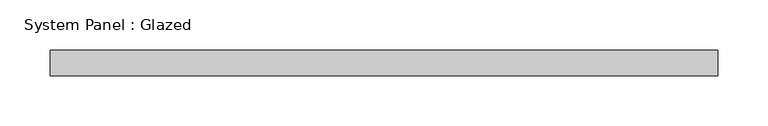
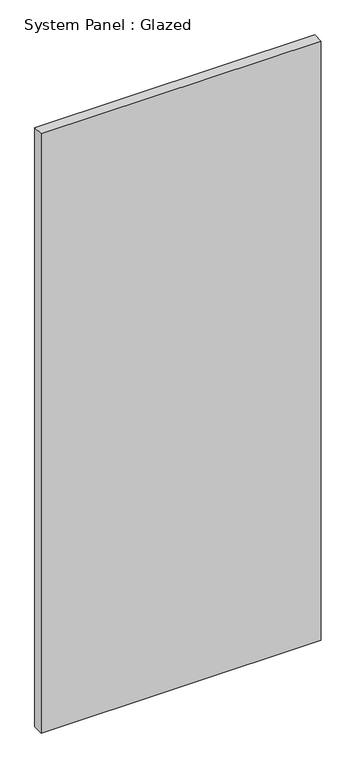
"""IFC4 building model written with IfcOpenShell, lengths in millimetres: plate geometry, System Panel : Glazed."""

from ifc_helpers import new_model, si_unit, origin, origin_with_axes, place, context, project, spatial, polyline, outline, extrude, source, transform, mapped, element, save


def system_panel_glazed_76c8377c(model_context):
    return source(origin(), model_context, "Body", "SweptSolid", [
        extrude(outline(polyline([(333.375, 19.05), (-333.375, 19.05), (-333.375, 44.45), (333.375, 44.45), (333.375, 19.05)])), origin_with_axes(), (0.0, 0.0, 1.0), 1507.2331996),
    ])


if __name__ == "__main__":
    model = new_model("IFC4")
    model_context = context("Model", 3, world=origin())
    ifc_project = project(units=[si_unit("LENGTHUNIT", "METRE", prefix="MILLI")], contexts=[model_context])
    site = spatial("IfcSite", under=ifc_project)
    building = spatial("IfcBuilding", under=site)
    placement = place(None, origin())
    system_panel_glazed_shape = system_panel_glazed_76c8377c(model_context)
    element("IfcPlate", 1, ObjectType="System Panel : Glazed", at=placement, inside=building, context=model_context, shape_type="MappedRepresentation", body=[
        mapped(system_panel_glazed_shape, transform((0.0, 0.0, 0.0), x_axis=(1.0, 0.0, 0.0), y_axis=(0.0, 1.0, 0.0), z_axis=(0.0, 0.0, 1.0))),
    ])
    save(model, "model.ifc")

# Revit data of these elements
# Type "System Panel : Glazed"
#   Construction Type Id = "GSP4R"
#   Analytic Construction = "1/8 in Pilkington single glazing"
#   Visual Light Transmittance = 0.9
#   Solar Heat Gain Coefficient = 0.86
#   Heat Transfer Coefficient (U) = 1.18115 BTU/(h·ft²·°F)
#   Define Thermal Properties by = 1
# Element 1 (IfcPlate, "System Panel : Glazed")
#   Materials on its faces: "Glass"
# Materials
#   "Glass": class "Glass", colour RGB 0 128 192, transparency 0.75, Description = "Soda Lime Glass", Cost = 0
